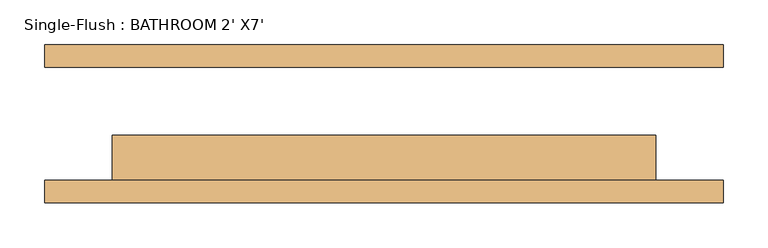
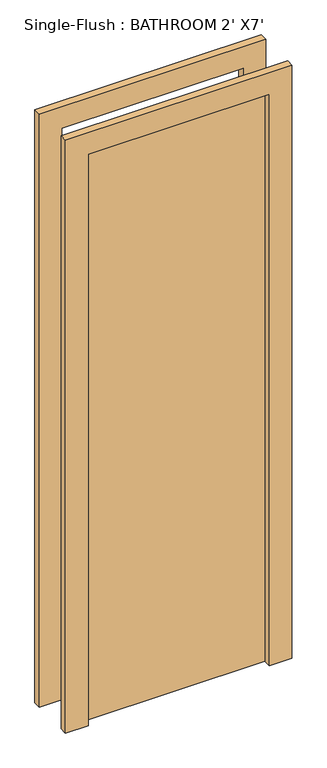
"""IFC4 building model written with IfcOpenShell, lengths in millimetres: door geometry, Single-Flush : BATHROOM 2' X7'."""

from ifc_helpers import new_model, si_unit, frame, origin, origin_with_axes, place, context, project, spatial, polyline, outline, extrude, source, transform, mapped, element, save


def single_flush_bathroom_2_x7_ccebbf4d(model_context):
    return source(origin(), model_context, "Body", "SweptSolid", [
        extrude(outline(polyline([(2108.2, -381.0), (0.0, -381.0), (0.0, -304.8), (2032.0, -304.8), (2032.0, 304.8), (0.0, 304.8), (0.0, 381.0), (2108.2, 381.0), (2108.2, -381.0)])), frame((0.0, -88.9, 0.0), z_axis=(0.0, 1.0, 0.0), x_axis=(0.0, 0.0, 1.0)), (0.0, 0.0, 1.0), 25.4),
        extrude(outline(polyline([(2108.2, 381.0), (2108.2, -381.0), (0.0, -381.0), (0.0, -304.8), (2032.0, -304.8), (2032.0, 304.8), (0.0, 304.8), (0.0, 381.0), (2108.2, 381.0)])), frame((0.0, 63.5, 0.0), z_axis=(0.0, 1.0, 0.0), x_axis=(0.0, 0.0, 1.0)), (0.0, 0.0, 1.0), 25.4),
        extrude(outline(polyline([(304.8, -12.7), (304.8, -63.5), (-304.8, -63.5), (-304.8, -12.7), (304.8, -12.7)])), origin_with_axes(), (0.0, 0.0, 1.0), 2032.0),
    ])


if __name__ == "__main__":
    model = new_model("IFC4")
    model_context = context("Model", 3, world=origin())
    ifc_project = project(units=[si_unit("LENGTHUNIT", "METRE", prefix="MILLI")], contexts=[model_context])
    site = spatial("IfcSite", under=ifc_project)
    building = spatial("IfcBuilding", under=site)
    placement = place(None, origin())
    single_flush_bathroom_2_x7_shape = single_flush_bathroom_2_x7_ccebbf4d(model_context)
    element("IfcDoor", 1, ObjectType="Single-Flush : BATHROOM 2' X7'", at=placement, inside=building, context=model_context, shape_type="MappedRepresentation", body=[
        mapped(single_flush_bathroom_2_x7_shape, transform((0.0, 0.0, 0.0), x_axis=(1.0, 0.0, 0.0), y_axis=(0.0, 1.0, 0.0), z_axis=(0.0, 0.0, 1.0))),
    ])
    save(model, "model.ifc")

# Revit data of these elements
# Type "Single-Flush : BATHROOM 2' X7'"
#   Type Mark = "12"
#   Construction Type Id = "MDOOR"
#   Assembly Code = "C1020"
#   Analytic Construction = "Metal"
#   Thickness = 0' - 2"
#   Heat Transfer Coefficient (U) = 0.651978 BTU/(h·ft²·°F)
#   Height = 6' - 8"
#   Trim Projection Ext = 0' - 1"
#   Trim Projection Int = 0' - 1"
#   Trim Width = 0' - 3"
#   Width = 2' - 0"
#   Define Thermal Properties by = 1
#   Door Material = Door - Panel
#   Frame Material = Door - Frame
#   Visual Light Transmittance = 0
#   Solar Heat Gain Coefficient = 0
#   Function = (empty or 0)
#   Wall Closure = (empty or 0)
# Element 1 (IfcDoor, "Single-Flush : BATHROOM 2' X7'")
#   Materials on its faces: "Door - Frame", "Door - Panel"
# Materials
#   "Door - Panel": class "Wood", colour RGB 210 159 95, transparency 0, Cost = 0
#   "Door - Frame": colour RGB 118 70 51, transparency 0, Cost = 0
